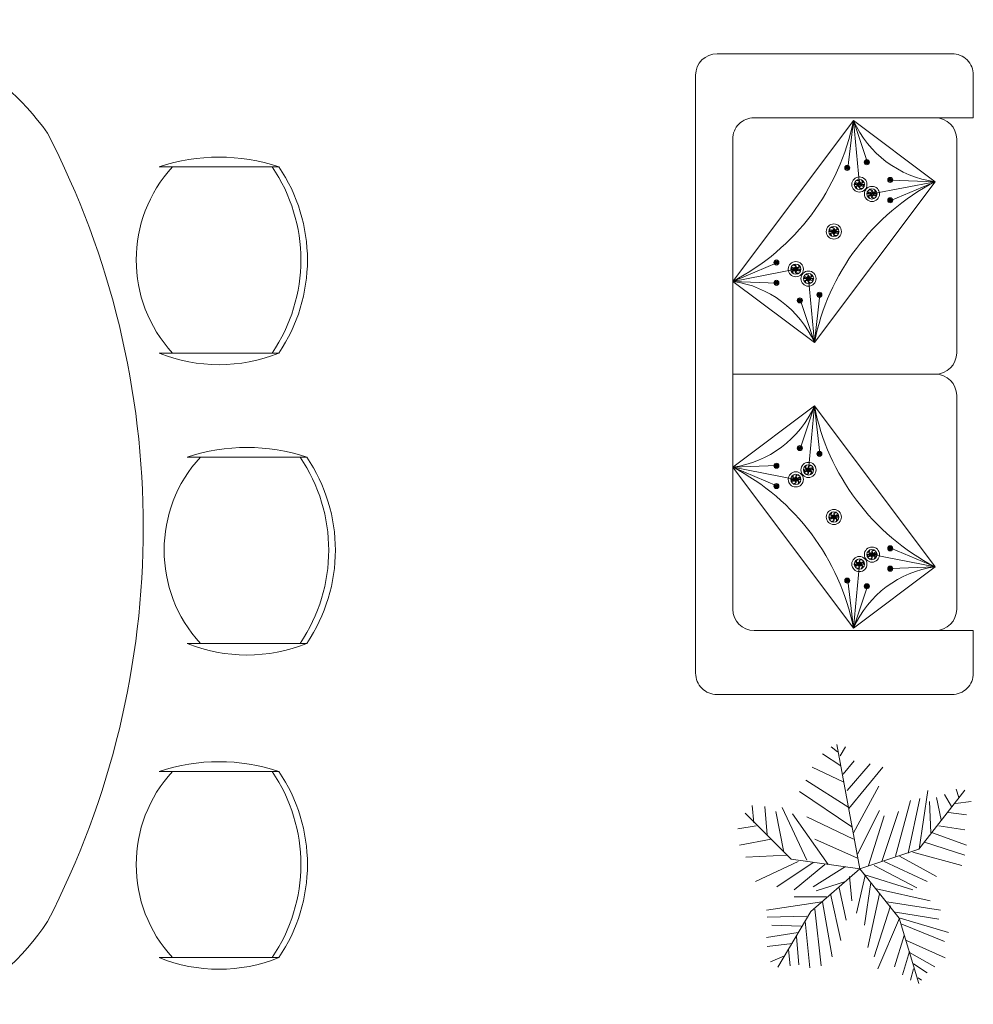
# Model space of a CAD drawing. Units: inches. Extents: x -61 to 1599, y -1316 to 257.
# Tile 170 of 204: x 1304 to 1393, y -937 to -845. Entities that reach past the tile are written whole.
import ezdxf

# ---------------------------------------------------------------- set-up
doc = ezdxf.new("R2010")
doc.units = ezdxf.units.IN
doc.header["$MEASUREMENT"] = 0
doc.layers.add('FUR', color=83, linetype='Continuous')
doc.layers.add('FURNITURE', color=83, linetype='Continuous', lineweight=18)

# ---------------------------------------------------------------- blocks, each defined once
blk = doc.blocks.new('*U264')
for p, q in [((-10.186, 53.64), (-13.084, 55.962)), ((0, 0), (-10.5, 57)), ((-9.099, 51.782), (-6.563, 55.962)), ((-8.737, 47.138), (-17.069, 52.711)), ((-7.288, 39.707), (-21.778, 46.673)), ((-7.65, 43.423), (-2.578, 49.46)), ((-5.839, 35.992), (4.667, 48.067)), ((-5.114, 27.632), (10.463, 46.673)), ((-5.114, 28.097), (-24.676, 40.636)), ((-2.941, 16.486), (8.652, 37.85)), ((44.153, 36.456), (45.239, 32.741)), ((-3.665, 19.273), (-27.574, 35.527)), ((22.055, 7.198), (27.489, 32.277)), ((27, 9), (48, 36)), ((27.127, 9.056), (31.112, 35.992)), ((35.096, 32.741), (37.27, 22.524)), ((38.719, 34.134), (41.979, 28.561)), ((-48.585, 21.131), (-49.309, 29.026)), ((-43.513, 28.561), (-42.427, 15.558)), ((-35.544, 28.097), (-24.314, 3.947)), ((16.259, 5.805), (23.142, 31.348)), ((31.836, 30.883), (32.561, 16.486)), ((43.791, 29.954), (51.036, 30.883)), ((-31.5, 4.5), (-52.5, 25.5)), ((-38.442, 26.239), (-34.819, 7.663)), ((-14.533, 2.09), (-30.834, 25.31)), ((-24.314, 23.917), (-2.941, 13.7)), ((-1.129, 6.734), (9.014, 26.704)), ((3.942, 1.625), (11.187, 24.381)), ((10.101, 3.483), (17.708, 26.239)), ((40.53, 25.775), (48.862, 24.846)), ((-47.498, 19.737), (-55.83, 18.344)), ((36.183, 19.737), (48.137, 17.88)), ((-40.615, 13.7), (-55.105, 10.913)), ((-20.691, 13.7), (-1.129, 4.876)), ((33.285, 16.486), (48.862, 10.913)), ((29.662, 12.307), (48.137, 6.269)), ((-33.37, 6.269), (-52.207, 5.34)), ((0, 0), (27, 9)), ((18.07, 5.805), (35.096, -3.483)), ((24.229, 7.663), (46.688, 1.625)), ((-28.299, 3.483), (-47.86, -5.805)), ((-21.416, 3.018), (-38.079, -8.128)), ((0, 0), (-31.5, 4.5)), ((-15.982, 2.09), (-30.11, -9.521)), ((0, 0), (-22.5, -19.5)), ((-6.563, 1.161), (-21.416, -8.128)), ((0, 0), (18, -22.5)), ((6.478, 1.625), (26.04, -8.592)), ((11.187, 3.483), (30.749, -5.805)), ((-4.752, -3.483), (-3.665, -14.629)), ((2.493, -3.019), (-1.491, -20.202)), ((1.769, -2.555), (24.229, -9.521)), ((-6.563, -5.805), (-19.967, -9.985)), ((-9.461, -8.592), (-6.201, -23.453)), ((5.029, -6.27), (2.131, -25.775)), ((-15.257, -12.772), (-30.11, -12.772)), ((-13.446, -11.378), (-8.737, -32.741)), ((9.014, -11.378), (3.58, -35.992)), ((7.565, -9.056), (32.198, -14.629)), ((-17.431, -15.094), (-42.789, -18.809)), ((-17.069, -15.094), (-12.721, -40.172)), ((14.085, -16.951), (6.478, -40.172)), ((12.274, -15.094), (36.907, -18.809)), ((-24.314, -21.596), (-42.427, -22.06)), ((-22.5, -19.5), (-37.5, -45)), ((-20.691, -18.345), (-17.793, -44.352)), ((18.07, -22.524), (8.289, -45.745)), ((16.259, -19.738), (36.183, -22.989)), ((18, -22.5), (27, -52.5)), ((18.433, -22.524), (40.53, -29.026)), ((-26.849, -26.24), (-40.253, -25.775)), ((-25.038, -23.918), (-22.865, -45.281)), ((19.157, -25.311), (38.719, -33.206)), ((-28.299, -29.026), (-42.789, -31.348)), ((-29.023, -30.884), (-27.936, -43.887)), ((20.244, -30.419), (15.897, -44.816)), ((-30.834, -34.135), (-42.427, -35.528)), ((21.331, -32.741), (39.081, -40.636)), ((-34.457, -39.708), (-40.978, -42.494)), ((-32.646, -36.921), (-31.921, -44.352)), ((22.78, -37.85), (19.519, -48.532)), ((22.78, -38.314), (34.372, -44.816)), ((24.591, -43.423), (30.749, -47.603)), ((24.591, -45.745), (23.142, -50.854)), ((26.764, -49.925), (28.213, -50.854))]:
    blk.add_line(p, q)
blk = doc.blocks.new('DINING-TABLE-OVAL')
for p, q in [((20.059, 34.258), (38.124, 65.35)), ((20.686, 45.856), (30.121, 61.177)), ((27.506, 37.684), (36.941, 53.006))]:
    blk.add_line(p, q)
for centre, radius, start, end in [((28.988, 70.072), 25.358, 35.51721, 144.48279), ((85.787, 47.892), 85.786, 154.51511, 205.48489), ((-21.854, 47.892), 80.449, 332.68902, 27.31098), ((28.988, 24.89), 24.889, 213.97533, 326.02467)]:
    blk.add_arc(centre, radius, start, end)
blk = doc.blocks.new('DINING-CHAIR')
for p, q in [((0.905, 2.156), (0.905, 13.354)), ((18.348, 2.156), (18.348, 13.354))]:
    blk.add_line(p, q)
for centre, radius, start, end in [((9.626, 0.517), 15.52, 55.80984, 124.19016), ((9.626, -0.104), 15.52, 55.80984, 124.19016), ((17.781, 7.755), 17.78, 161.64548, 198.35452), ((4.514, 7.755), 14.923, 337.96463, 22.03537), ((9.626, 12.869), 12.868, 227.33204, 312.66796)]:
    blk.add_arc(centre, radius, start, end)
blk = doc.blocks.new('*U160')
at = {"layer": 'FUR'}
blk.add_open_spline([(0.005, 0.08), (-0.03, 0.048), (-0.098, -0.015), (0.075, -0.018), (0.024, -0.063), (0.005, -0.08)], degree=3, knots=[0, 0, 0, 0, 0.0954578, 0.1898773, 0.2470677, 0.2470677, 0.2470677, 0.2470677], dxfattribs=at)
blk = doc.blocks.new('*U161')
at = {"layer": 'FUR', "transparency": 16777216}
for p, rotation in [((222.173, -79.977), 60), ((222.178, -80.056), 120), ((222.25, -80.092), 180), ((222.312, -79.968), 300), ((222.317, -80.048), 240)]:
    blk.add_blockref('*U160', p, dxfattribs=dict(at, rotation=rotation))
blk.add_blockref('*U160', (222.24, -79.932), dxfattribs=at)
blk = doc.blocks.new('*U172')
at = {"layer": 'FUR'}
blk.add_open_spline([(0.005, 0.08), (-0.03, 0.048), (-0.098, -0.015), (0.075, -0.018), (0.024, -0.063), (0.005, -0.08)], degree=3, knots=[0, 0, 0, 0, 0.0954578, 0.1898773, 0.2470677, 0.2470677, 0.2470677, 0.2470677], dxfattribs=at)
blk = doc.blocks.new('*U173')
at = {"layer": 'FUR', "transparency": 16777216}
for p, rotation in [((222.173, -79.977), 60), ((222.178, -80.056), 120), ((222.25, -80.092), 180), ((222.312, -79.968), 300), ((222.317, -80.048), 240)]:
    blk.add_blockref('*U172', p, dxfattribs=dict(at, rotation=rotation))
blk.add_blockref('*U172', (222.24, -79.932), dxfattribs=at)
blk = doc.blocks.new('*U186')
at = {"layer": 'FUR'}
blk.add_open_spline([(0.005, 0.08), (-0.03, 0.048), (-0.098, -0.015), (0.075, -0.018), (0.024, -0.063), (0.005, -0.08)], degree=3, knots=[0, 0, 0, 0, 0.0954578, 0.1898773, 0.2470677, 0.2470677, 0.2470677, 0.2470677], dxfattribs=at)
blk = doc.blocks.new('*U187')
at = {"layer": 'FUR', "transparency": 16777216}
for p, rotation in [((222.173, -79.977), 60), ((222.178, -80.056), 120), ((222.25, -80.092), 180), ((222.312, -79.968), 300), ((222.317, -80.048), 240)]:
    blk.add_blockref('*U186', p, dxfattribs=dict(at, rotation=rotation))
blk.add_blockref('*U186', (222.24, -79.932), dxfattribs=at)
blk = doc.blocks.new('*U198')
at = {"layer": 'FUR'}
blk.add_open_spline([(0.005, 0.08), (-0.03, 0.048), (-0.098, -0.015), (0.075, -0.018), (0.024, -0.063), (0.005, -0.08)], degree=3, knots=[0, 0, 0, 0, 0.0954578, 0.1898773, 0.2470677, 0.2470677, 0.2470677, 0.2470677], dxfattribs=at)
blk = doc.blocks.new('*U199')
at = {"layer": 'FUR', "transparency": 16777216}
for p, rotation in [((222.173, -79.977), 60), ((222.178, -80.056), 120), ((222.25, -80.092), 180), ((222.312, -79.968), 300), ((222.317, -80.048), 240)]:
    blk.add_blockref('*U198', p, dxfattribs=dict(at, rotation=rotation))
blk.add_blockref('*U198', (222.24, -79.932), dxfattribs=at)
blk = doc.blocks.new('*U184')
at = {"layer": 'FUR'}
blk.add_open_spline([(0.015, 0.238), (-0.088, 0.143), (-0.292, -0.045), (0.224, -0.053), (0.072, -0.187), (0.015, -0.238)], degree=3, knots=[0, 0, 0, 0, 0.2846533, 0.5662105, 0.736751, 0.736751, 0.736751, 0.736751], dxfattribs=at)
blk = doc.blocks.new('*U159')
at = {"layer": 'FUR', "transparency": 16777216}
for p, rotation in [((662.517, -238.489), 60), ((662.531, -238.727), 120), ((662.745, -238.833), 180), ((662.929, -238.463), 300), ((662.944, -238.702), 240)]:
    blk.add_blockref('*U184', p, dxfattribs=dict(at, rotation=rotation))
blk.add_blockref('*U184', (662.716, -238.357), dxfattribs=at)
blk = doc.blocks.new('*U210')
at = {"layer": 'FUR'}
blk.add_open_spline([(0.015, 0.238), (-0.088, 0.143), (-0.292, -0.045), (0.224, -0.053), (0.072, -0.187), (0.015, -0.238)], degree=3, knots=[0, 0, 0, 0, 0.2846533, 0.5662105, 0.736751, 0.736751, 0.736751, 0.736751], dxfattribs=at)
blk = doc.blocks.new('*U185')
at = {"layer": 'FUR', "transparency": 16777216}
for p, rotation in [((662.517, -238.489), 60), ((662.531, -238.727), 120), ((662.745, -238.833), 180), ((662.929, -238.463), 300), ((662.944, -238.702), 240)]:
    blk.add_blockref('*U210', p, dxfattribs=dict(at, rotation=rotation))
blk.add_blockref('*U210', (662.716, -238.357), dxfattribs=at)
blk = doc.blocks.new('*U174')
at = {"layer": 'FUR'}
blk.add_open_spline([(0.005, 0.08), (-0.03, 0.048), (-0.098, -0.015), (0.075, -0.018), (0.024, -0.063), (0.005, -0.08)], degree=3, knots=[0, 0, 0, 0, 0.0954578, 0.1898773, 0.2470677, 0.2470677, 0.2470677, 0.2470677], dxfattribs=at)
blk = doc.blocks.new('*U175')
at = {"layer": 'FUR', "transparency": 16777216}
for p, rotation in [((222.173, -79.977), 60), ((222.178, -80.056), 120), ((222.25, -80.092), 180), ((222.312, -79.968), 300), ((222.317, -80.048), 240)]:
    blk.add_blockref('*U174', p, dxfattribs=dict(at, rotation=rotation))
blk.add_blockref('*U174', (222.24, -79.932), dxfattribs=at)
blk = doc.blocks.new('*U200')
at = {"layer": 'FUR'}
blk.add_open_spline([(0.005, 0.08), (-0.03, 0.048), (-0.098, -0.015), (0.075, -0.018), (0.024, -0.063), (0.005, -0.08)], degree=3, knots=[0, 0, 0, 0, 0.0954578, 0.1898773, 0.2470677, 0.2470677, 0.2470677, 0.2470677], dxfattribs=at)
blk = doc.blocks.new('*U201')
at = {"layer": 'FUR', "transparency": 16777216}
for p, rotation in [((222.173, -79.977), 60), ((222.178, -80.056), 120), ((222.25, -80.092), 180), ((222.312, -79.968), 300), ((222.317, -80.048), 240)]:
    blk.add_blockref('*U200', p, dxfattribs=dict(at, rotation=rotation))
blk.add_blockref('*U200', (222.24, -79.932), dxfattribs=at)
blk = doc.blocks.new('*U168')
at = {"layer": 'FUR'}
blk.add_open_spline([(0.015, 0.238), (-0.088, 0.143), (-0.292, -0.045), (0.224, -0.053), (0.072, -0.187), (0.015, -0.238)], degree=3, knots=[0, 0, 0, 0, 0.2846533, 0.5662105, 0.736751, 0.736751, 0.736751, 0.736751], dxfattribs=at)
blk = doc.blocks.new('*U169')
at = {"layer": 'FUR', "transparency": 16777216}
for p, rotation in [((662.517, -238.489), 60), ((662.531, -238.727), 120), ((662.745, -238.833), 180), ((662.929, -238.463), 300), ((662.944, -238.702), 240)]:
    blk.add_blockref('*U168', p, dxfattribs=dict(at, rotation=rotation))
blk.add_blockref('*U168', (662.716, -238.357), dxfattribs=at)
blk = doc.blocks.new('*U194')
at = {"layer": 'FUR'}
blk.add_open_spline([(0.015, 0.238), (-0.088, 0.143), (-0.292, -0.045), (0.224, -0.053), (0.072, -0.187), (0.015, -0.238)], degree=3, knots=[0, 0, 0, 0, 0.2846533, 0.5662105, 0.736751, 0.736751, 0.736751, 0.736751], dxfattribs=at)
blk = doc.blocks.new('*U195')
at = {"layer": 'FUR', "transparency": 16777216}
for p, rotation in [((662.517, -238.489), 60), ((662.531, -238.727), 120), ((662.745, -238.833), 180), ((662.929, -238.463), 300), ((662.944, -238.702), 240)]:
    blk.add_blockref('*U194', p, dxfattribs=dict(at, rotation=rotation))
blk.add_blockref('*U194', (662.716, -238.357), dxfattribs=at)
blk = doc.blocks.new('*U176')
at = {"layer": 'FUR'}
blk.add_open_spline([(0.005, 0.08), (-0.03, 0.048), (-0.098, -0.015), (0.075, -0.018), (0.024, -0.063), (0.005, -0.08)], degree=3, knots=[0, 0, 0, 0, 0.0954578, 0.1898773, 0.2470677, 0.2470677, 0.2470677, 0.2470677], dxfattribs=at)
blk = doc.blocks.new('*U177')
at = {"layer": 'FUR', "transparency": 16777216}
for p, rotation in [((222.173, -79.977), 60), ((222.178, -80.056), 120), ((222.25, -80.092), 180), ((222.312, -79.968), 300), ((222.317, -80.048), 240)]:
    blk.add_blockref('*U176', p, dxfattribs=dict(at, rotation=rotation))
blk.add_blockref('*U176', (222.24, -79.932), dxfattribs=at)
blk = doc.blocks.new('*U202')
at = {"layer": 'FUR'}
blk.add_open_spline([(0.005, 0.08), (-0.03, 0.048), (-0.098, -0.015), (0.075, -0.018), (0.024, -0.063), (0.005, -0.08)], degree=3, knots=[0, 0, 0, 0, 0.0954578, 0.1898773, 0.2470677, 0.2470677, 0.2470677, 0.2470677], dxfattribs=at)
blk = doc.blocks.new('*U203')
at = {"layer": 'FUR', "transparency": 16777216}
for p, rotation in [((222.173, -79.977), 60), ((222.178, -80.056), 120), ((222.25, -80.092), 180), ((222.312, -79.968), 300), ((222.317, -80.048), 240)]:
    blk.add_blockref('*U202', p, dxfattribs=dict(at, rotation=rotation))
blk.add_blockref('*U202', (222.24, -79.932), dxfattribs=at)
blk = doc.blocks.new('*U170')
at = {"layer": 'FUR'}
blk.add_open_spline([(0.015, 0.238), (-0.088, 0.143), (-0.292, -0.045), (0.224, -0.053), (0.072, -0.187), (0.015, -0.238)], degree=3, knots=[0, 0, 0, 0, 0.2846533, 0.5662105, 0.736751, 0.736751, 0.736751, 0.736751], dxfattribs=at)
blk = doc.blocks.new('*U171')
at = {"layer": 'FUR', "transparency": 16777216}
for p, rotation in [((662.517, -238.489), 60), ((662.531, -238.727), 120), ((662.745, -238.833), 180), ((662.929, -238.463), 300), ((662.944, -238.702), 240)]:
    blk.add_blockref('*U170', p, dxfattribs=dict(at, rotation=rotation))
blk.add_blockref('*U170', (662.716, -238.357), dxfattribs=at)
blk = doc.blocks.new('*U196')
at = {"layer": 'FUR'}
blk.add_open_spline([(0.015, 0.238), (-0.088, 0.143), (-0.292, -0.045), (0.224, -0.053), (0.072, -0.187), (0.015, -0.238)], degree=3, knots=[0, 0, 0, 0, 0.2846533, 0.5662105, 0.736751, 0.736751, 0.736751, 0.736751], dxfattribs=at)
blk = doc.blocks.new('*U197')
at = {"layer": 'FUR', "transparency": 16777216}
for p, rotation in [((662.517, -238.489), 60), ((662.531, -238.727), 120), ((662.745, -238.833), 180), ((662.929, -238.463), 300), ((662.944, -238.702), 240)]:
    blk.add_blockref('*U196', p, dxfattribs=dict(at, rotation=rotation))
blk.add_blockref('*U196', (662.716, -238.357), dxfattribs=at)
blk = doc.blocks.new('*U164')
at = {"layer": 'FUR'}
blk.add_open_spline([(0.005, 0.08), (-0.03, 0.048), (-0.098, -0.015), (0.075, -0.018), (0.024, -0.063), (0.005, -0.08)], degree=3, knots=[0, 0, 0, 0, 0.0954578, 0.1898773, 0.2470677, 0.2470677, 0.2470677, 0.2470677], dxfattribs=at)
blk = doc.blocks.new('*U165')
at = {"layer": 'FUR', "transparency": 16777216}
for p, rotation in [((222.173, -79.977), 60), ((222.178, -80.056), 120), ((222.25, -80.092), 180), ((222.312, -79.968), 300), ((222.317, -80.048), 240)]:
    blk.add_blockref('*U164', p, dxfattribs=dict(at, rotation=rotation))
blk.add_blockref('*U164', (222.24, -79.932), dxfattribs=at)
blk = doc.blocks.new('*U190')
at = {"layer": 'FUR'}
blk.add_open_spline([(0.005, 0.08), (-0.03, 0.048), (-0.098, -0.015), (0.075, -0.018), (0.024, -0.063), (0.005, -0.08)], degree=3, knots=[0, 0, 0, 0, 0.0954578, 0.1898773, 0.2470677, 0.2470677, 0.2470677, 0.2470677], dxfattribs=at)
blk = doc.blocks.new('*U191')
at = {"layer": 'FUR', "transparency": 16777216}
for p, rotation in [((222.173, -79.977), 60), ((222.178, -80.056), 120), ((222.25, -80.092), 180), ((222.312, -79.968), 300), ((222.317, -80.048), 240)]:
    blk.add_blockref('*U190', p, dxfattribs=dict(at, rotation=rotation))
blk.add_blockref('*U190', (222.24, -79.932), dxfattribs=at)
blk = doc.blocks.new('*U183')
at = {"layer": 'FUR'}
blk.add_open_spline([(0.015, 0.238), (-0.088, 0.143), (-0.292, -0.045), (0.224, -0.053), (0.072, -0.187), (0.015, -0.238)], degree=3, knots=[0, 0, 0, 0, 0.2846533, 0.5662105, 0.736751, 0.736751, 0.736751, 0.736751], dxfattribs=at)
blk = doc.blocks.new('*U162')
at = {"layer": 'FUR', "transparency": 16777216}
for p, rotation in [((662.517, -238.489), 60), ((662.531, -238.727), 120), ((662.745, -238.833), 180), ((662.929, -238.463), 300), ((662.944, -238.702), 240)]:
    blk.add_blockref('*U183', p, dxfattribs=dict(at, rotation=rotation))
blk.add_blockref('*U183', (662.716, -238.357), dxfattribs=at)
blk = doc.blocks.new('*U209')
at = {"layer": 'FUR'}
blk.add_open_spline([(0.015, 0.238), (-0.088, 0.143), (-0.292, -0.045), (0.224, -0.053), (0.072, -0.187), (0.015, -0.238)], degree=3, knots=[0, 0, 0, 0, 0.2846533, 0.5662105, 0.736751, 0.736751, 0.736751, 0.736751], dxfattribs=at)
blk = doc.blocks.new('*U188')
at = {"layer": 'FUR', "transparency": 16777216}
for p, rotation in [((662.517, -238.489), 60), ((662.531, -238.727), 120), ((662.745, -238.833), 180), ((662.929, -238.463), 300), ((662.944, -238.702), 240)]:
    blk.add_blockref('*U209', p, dxfattribs=dict(at, rotation=rotation))
blk.add_blockref('*U209', (662.716, -238.357), dxfattribs=at)
blk = doc.blocks.new('*U182')
at = {"layer": 'FUR'}
blk.add_open_spline([(0.005, 0.08), (-0.03, 0.048), (-0.098, -0.015), (0.075, -0.018), (0.024, -0.063), (0.005, -0.08)], degree=3, knots=[0, 0, 0, 0, 0.0954578, 0.1898773, 0.2470677, 0.2470677, 0.2470677, 0.2470677], dxfattribs=at)
blk = doc.blocks.new('*U163')
at = {"layer": 'FUR', "transparency": 16777216}
for p, rotation in [((222.173, -79.977), 60), ((222.178, -80.056), 120), ((222.25, -80.092), 180), ((222.312, -79.968), 300), ((222.317, -80.048), 240)]:
    blk.add_blockref('*U182', p, dxfattribs=dict(at, rotation=rotation))
blk.add_blockref('*U182', (222.24, -79.932), dxfattribs=at)
blk = doc.blocks.new('*U208')
at = {"layer": 'FUR'}
blk.add_open_spline([(0.005, 0.08), (-0.03, 0.048), (-0.098, -0.015), (0.075, -0.018), (0.024, -0.063), (0.005, -0.08)], degree=3, knots=[0, 0, 0, 0, 0.0954578, 0.1898773, 0.2470677, 0.2470677, 0.2470677, 0.2470677], dxfattribs=at)
blk = doc.blocks.new('*U189')
at = {"layer": 'FUR', "transparency": 16777216}
for p, rotation in [((222.173, -79.977), 60), ((222.178, -80.056), 120), ((222.25, -80.092), 180), ((222.312, -79.968), 300), ((222.317, -80.048), 240)]:
    blk.add_blockref('*U208', p, dxfattribs=dict(at, rotation=rotation))
blk.add_blockref('*U208', (222.24, -79.932), dxfattribs=at)
blk = doc.blocks.new('*U166')
at = {"layer": 'FUR'}
blk.add_open_spline([(0.015, 0.238), (-0.088, 0.143), (-0.292, -0.045), (0.224, -0.053), (0.072, -0.187), (0.015, -0.238)], degree=3, knots=[0, 0, 0, 0, 0.2846533, 0.5662105, 0.736751, 0.736751, 0.736751, 0.736751], dxfattribs=at)
blk = doc.blocks.new('*U167')
at = {"layer": 'FUR', "transparency": 16777216}
for p, rotation in [((662.517, -238.489), 60), ((662.531, -238.727), 120), ((662.745, -238.833), 180), ((662.929, -238.463), 300), ((662.944, -238.702), 240)]:
    blk.add_blockref('*U166', p, dxfattribs=dict(at, rotation=rotation))
blk.add_blockref('*U166', (662.716, -238.357), dxfattribs=at)
blk = doc.blocks.new('*U192')
at = {"layer": 'FUR'}
blk.add_open_spline([(0.015, 0.238), (-0.088, 0.143), (-0.292, -0.045), (0.224, -0.053), (0.072, -0.187), (0.015, -0.238)], degree=3, knots=[0, 0, 0, 0, 0.2846533, 0.5662105, 0.736751, 0.736751, 0.736751, 0.736751], dxfattribs=at)
blk = doc.blocks.new('*U193')
at = {"layer": 'FUR', "transparency": 16777216}
for p, rotation in [((662.517, -238.489), 60), ((662.531, -238.727), 120), ((662.745, -238.833), 180), ((662.929, -238.463), 300), ((662.944, -238.702), 240)]:
    blk.add_blockref('*U192', p, dxfattribs=dict(at, rotation=rotation))
blk.add_blockref('*U192', (662.716, -238.357), dxfattribs=at)
blk = doc.blocks.new('*U178')
at = {"layer": 'FUR'}
blk.add_open_spline([(0.005, 0.08), (-0.03, 0.048), (-0.098, -0.015), (0.075, -0.018), (0.024, -0.063), (0.005, -0.08)], degree=3, knots=[0, 0, 0, 0, 0.0954578, 0.1898773, 0.2470677, 0.2470677, 0.2470677, 0.2470677], dxfattribs=at)
blk = doc.blocks.new('*U179')
at = {"layer": 'FUR', "transparency": 16777216}
for p, rotation in [((222.173, -79.977), 60), ((222.178, -80.056), 120), ((222.25, -80.092), 180), ((222.312, -79.968), 300), ((222.317, -80.048), 240)]:
    blk.add_blockref('*U178', p, dxfattribs=dict(at, rotation=rotation))
blk.add_blockref('*U178', (222.24, -79.932), dxfattribs=at)
blk = doc.blocks.new('*U180')
at = {"layer": 'FUR'}
blk.add_open_spline([(0.005, 0.08), (-0.03, 0.048), (-0.098, -0.015), (0.075, -0.018), (0.024, -0.063), (0.005, -0.08)], degree=3, knots=[0, 0, 0, 0, 0.0954578, 0.1898773, 0.2470677, 0.2470677, 0.2470677, 0.2470677], dxfattribs=at)
blk = doc.blocks.new('*U181')
at = {"layer": 'FUR', "transparency": 16777216}
for p, rotation in [((222.173, -79.977), 60), ((222.178, -80.056), 120), ((222.25, -80.092), 180), ((222.312, -79.968), 300), ((222.317, -80.048), 240)]:
    blk.add_blockref('*U180', p, dxfattribs=dict(at, rotation=rotation))
blk.add_blockref('*U180', (222.24, -79.932), dxfattribs=at)
blk = doc.blocks.new('*U204')
at = {"layer": 'FUR'}
blk.add_open_spline([(0.005, 0.08), (-0.03, 0.048), (-0.098, -0.015), (0.075, -0.018), (0.024, -0.063), (0.005, -0.08)], degree=3, knots=[0, 0, 0, 0, 0.0954578, 0.1898773, 0.2470677, 0.2470677, 0.2470677, 0.2470677], dxfattribs=at)
blk = doc.blocks.new('*U205')
at = {"layer": 'FUR', "transparency": 16777216}
for p, rotation in [((222.173, -79.977), 60), ((222.178, -80.056), 120), ((222.25, -80.092), 180), ((222.312, -79.968), 300), ((222.317, -80.048), 240)]:
    blk.add_blockref('*U204', p, dxfattribs=dict(at, rotation=rotation))
blk.add_blockref('*U204', (222.24, -79.932), dxfattribs=at)
blk = doc.blocks.new('*U206')
at = {"layer": 'FUR'}
blk.add_open_spline([(0.005, 0.08), (-0.03, 0.048), (-0.098, -0.015), (0.075, -0.018), (0.024, -0.063), (0.005, -0.08)], degree=3, knots=[0, 0, 0, 0, 0.0954578, 0.1898773, 0.2470677, 0.2470677, 0.2470677, 0.2470677], dxfattribs=at)
blk = doc.blocks.new('*U207')
at = {"layer": 'FUR', "transparency": 16777216}
for p, rotation in [((222.173, -79.977), 60), ((222.178, -80.056), 120), ((222.25, -80.092), 180), ((222.312, -79.968), 300), ((222.317, -80.048), 240)]:
    blk.add_blockref('*U206', p, dxfattribs=dict(at, rotation=rotation))
blk.add_blockref('*U206', (222.24, -79.932), dxfattribs=at)
blk = doc.blocks.new('SOFA-LOVESEAT')
for p, q in [((22.442, 54), (5.47, 54)), ((14.776, 53.751), (14.253, 49.285)), ((14.776, 53.751), (15.332, 47.757)), ((14.776, 53.751), (16.081, 49.817)), ((22.442, 54), (26, 54)), ((3.47, 8), (3.47, 52)), ((24.442, 52), (24.442, 32)), ((16.029, 49.837), (15.869, 49.837)), ((16.029, 49.837), (16.189, 49.837)), ((14.201, 49.305), (14.041, 49.305)), ((14.201, 49.305), (14.36, 49.305)), ((22.422, 48.013), (16.511, 46.872)), ((18.228, 48.187), (18.068, 48.187)), ((18.228, 48.187), (18.388, 48.187)), ((22.422, 48.013), (18.28, 48.167)), ((22.422, 48.013), (18.28, 46.263)), ((15.332, 47.757), (14.855, 47.757)), ((15.332, 47.757), (15.808, 47.757)), ((16.511, 46.872), (16.035, 46.872)), ((16.511, 46.872), (16.988, 46.872)), ((18.228, 46.282), (18.068, 46.282)), ((18.228, 46.282), (18.388, 46.282)), ((12.946, 43.35), (12.47, 43.35)), ((12.946, 43.35), (13.423, 43.35)), ((3.47, 38.686), (7.612, 40.436)), ((3.47, 38.686), (9.381, 39.828)), ((7.56, 40.455), (7.4, 40.455)), ((7.56, 40.455), (7.719, 40.455)), ((9.381, 39.828), (8.904, 39.828)), ((9.381, 39.828), (9.857, 39.828)), ((10.561, 38.942), (10.084, 38.942)), ((11.116, 32.948), (10.561, 38.942)), ((10.561, 38.942), (11.037, 38.942)), ((3.47, 38.686), (7.612, 38.532)), ((7.56, 38.551), (7.4, 38.551)), ((7.56, 38.551), (7.719, 38.551)), ((9.759, 36.901), (9.599, 36.901)), ((9.759, 36.901), (9.918, 36.901)), ((11.116, 32.948), (9.811, 36.882)), ((11.116, 32.948), (11.639, 37.414)), ((11.587, 37.433), (11.427, 37.433)), ((11.587, 37.433), (11.747, 37.433)), ((22.442, 30), (3.47, 30)), ((22.442, 30), (22.442, 30)), ((24.442, 8), (24.442, 28)), ((11.116, 27.026), (9.811, 23.092)), ((11.116, 27.026), (10.561, 21.032)), ((11.116, 27.026), (11.639, 22.56)), ((9.759, 23.073), (9.599, 23.073)), ((9.759, 23.073), (9.918, 23.073)), ((11.587, 22.541), (11.427, 22.541)), ((11.587, 22.541), (11.747, 22.541)), ((3.47, 21.288), (7.612, 21.442)), ((3.47, 21.288), (9.381, 20.146)), ((3.47, 21.288), (7.612, 19.538)), ((7.56, 21.423), (7.4, 21.423)), ((7.56, 21.423), (7.719, 21.423)), ((10.561, 21.032), (10.084, 21.032)), ((10.561, 21.032), (11.037, 21.032)), ((7.56, 19.518), (7.4, 19.518)), ((7.56, 19.518), (7.719, 19.518)), ((9.381, 20.146), (8.904, 20.146)), ((9.381, 20.146), (9.857, 20.146)), ((12.946, 16.624), (12.47, 16.624)), ((12.946, 16.624), (13.423, 16.624)), ((16.511, 13.102), (16.035, 13.102)), ((22.422, 11.961), (16.511, 13.102)), ((16.511, 13.102), (16.988, 13.102)), ((18.228, 13.691), (18.068, 13.691)), ((18.228, 13.691), (18.388, 13.691)), ((22.422, 11.961), (18.28, 13.711)), ((14.776, 6.223), (15.332, 12.217)), ((15.332, 12.217), (14.855, 12.217)), ((15.332, 12.217), (15.808, 12.217)), ((18.228, 11.787), (18.068, 11.787)), ((18.228, 11.787), (18.388, 11.787)), ((22.422, 11.961), (18.28, 11.807)), ((14.201, 10.669), (14.041, 10.669)), ((14.201, 10.669), (14.36, 10.669)), ((14.776, 6.223), (14.253, 10.689)), ((14.776, 6.223), (16.081, 10.156)), ((16.029, 10.137), (15.869, 10.137)), ((16.029, 10.137), (16.189, 10.137)), ((22.442, 6), (5.47, 6)), ((22.442, 6), (26, 6))]:
    blk.add_line(p, q)
blk.add_lwpolyline([(26, 6), (26, 2, -0.414214), (24, 0), (2, 0, -0.414214), (0, 2), (0, 58, -0.414213), (2, 60), (24, 60, -0.414214), (26, 58), (26, 54)], format="xyb")
for points in [[(11.116, 32.948), (22.422, 48.013), (14.776, 53.751), (3.47, 38.686)], [(11.116, 27.026), (22.422, 11.961), (14.776, 6.223), (3.47, 21.288)]]:
    blk.add_lwpolyline(points, close=True)
for centre, radius in [((16.029, 49.837), 0.238), ((16.029, 49.837), 0.16), ((14.201, 49.305), 0.238), ((14.201, 49.305), 0.16), ((15.332, 47.757), 0.71), ((15.332, 47.757), 0.476), ((18.228, 48.187), 0.238), ((18.228, 48.187), 0.16), ((16.511, 46.872), 0.71), ((16.511, 46.872), 0.476), ((18.228, 46.282), 0.238), ((18.228, 46.282), 0.16), ((12.946, 43.35), 0.71), ((12.946, 43.35), 0.476), ((7.56, 40.455), 0.238), ((7.56, 40.455), 0.16), ((9.381, 39.828), 0.71), ((9.381, 39.828), 0.476), ((10.561, 38.942), 0.71), ((7.56, 38.551), 0.238), ((10.561, 38.942), 0.476), ((7.56, 38.551), 0.16), ((9.759, 36.901), 0.238), ((9.759, 36.901), 0.16), ((11.587, 37.433), 0.238), ((11.587, 37.433), 0.16), ((9.759, 23.073), 0.238), ((9.759, 23.073), 0.16), ((11.587, 22.541), 0.238), ((11.587, 22.541), 0.16), ((7.56, 21.423), 0.238), ((7.56, 21.423), 0.16), ((10.561, 21.032), 0.71), ((10.561, 21.032), 0.476), ((9.381, 20.146), 0.71), ((9.381, 20.146), 0.476), ((7.56, 19.518), 0.238), ((7.56, 19.518), 0.16), ((12.946, 16.624), 0.71), ((12.946, 16.624), 0.476), ((18.228, 13.691), 0.238), ((18.228, 13.691), 0.16), ((15.332, 12.217), 0.71), ((16.511, 13.102), 0.71), ((16.511, 13.102), 0.476), ((15.332, 12.217), 0.476), ((18.228, 11.787), 0.238), ((18.228, 11.787), 0.16), ((14.201, 10.669), 0.238), ((14.201, 10.669), 0.16), ((16.029, 10.137), 0.238), ((16.029, 10.137), 0.16)]:
    blk.add_circle(centre, radius)
for centre, radius, start, end in [((5.47, 52), 2, 90, 180.00002), ((-6.541, 57.974), 21.731, 297.43166, 348.79559), ((23.745, 57.74), 9.816, 203.97425, 262.253), ((22.442, 52), 2, 0, 90), ((32.433, 28.726), 21.731, 117.43166, 168.79559), ((2.147, 28.96), 9.816, 23.97425, 82.253), ((22.442, 32), 2, 270, 0), ((22.442, 28), 2, 0, 90), ((2.147, 31.014), 9.816, 277.74703, 336.02578), ((32.433, 31.248), 21.731, 191.20444, 242.56837), ((-6.541, 2), 21.731, 11.20444, 62.56837), ((23.745, 2.234), 9.816, 97.74703, 156.02578), ((5.47, 8), 2, 180.00002, 270), ((22.442, 8), 2, 270, 0)]:
    blk.add_arc(centre, radius, start, end)
at = {"xscale": -1, "rotation": 90.00003000000098}
for name, p in [('*U189', (-63.984, 272.082)), ('*U191', (-65.812, 271.55)), ('*U188', (-223.264, 710.487)), ('*U205', (-61.785, 270.431)), ('*U193', (-222.084, 709.602)), ('*U207', (-61.785, 268.527)), ('*U197', (-225.649, 706.08)), ('*U187', (-72.453, 262.7)), ('*U185', (-229.215, 702.558)), ('*U199', (-72.453, 260.796)), ('*U195', (-228.035, 701.672)), ('*U201', (-70.254, 259.146)), ('*U203', (-68.426, 259.678))]:
    blk.add_blockref(name, p, dxfattribs=at)
at = {"rotation": 90}
for name, p in [('*U175', (-70.254, -199.172)), ('*U177', (-68.425, -199.704)), ('*U173', (-72.453, -200.822)), ('*U169', (-228.034, -641.698)), ('*U159', (-229.214, -642.584)), ('*U161', (-72.453, -202.727)), ('*U171', (-225.649, -646.106)), ('*U181', (-61.785, -208.554)), ('*U167', (-222.084, -649.628)), ('*U162', (-223.264, -650.513)), ('*U179', (-61.785, -210.458)), ('*U165', (-65.812, -211.576)), ('*U163', (-63.983, -212.108))]:
    blk.add_blockref(name, p, dxfattribs=at)

msp = doc.modelspace()

# ---------------------------------------------------------------- block references
at = {"layer": 'FURNITURE'}
for name, p in [('DINING-TABLE-OVAL', (1256.634, -940.4721)), ('SOFA-LOVESEAT', (1366.9518, -908.2291))]:
    msp.add_blockref(name, p, dxfattribs=at)
for p, rotation in [((1314.562, -857.909), 270.000000000001), ((1317.1761, -885.0906), 269.9999999999969), ((1314.562, -914.5159), 270.0000000000014)]:
    msp.add_blockref('DINING-CHAIR', p, dxfattribs=dict(at, rotation=rotation))
at = {"layer": 'FURNITURE', "xscale": 0.2045054661246738, "yscale": 0.2045054661246738, "zscale": 0.2045054661246738}
msp.add_blockref('*U264', (1382.3297, -924.5581), dxfattribs=at)

doc.saveas('drawing.dxf')
